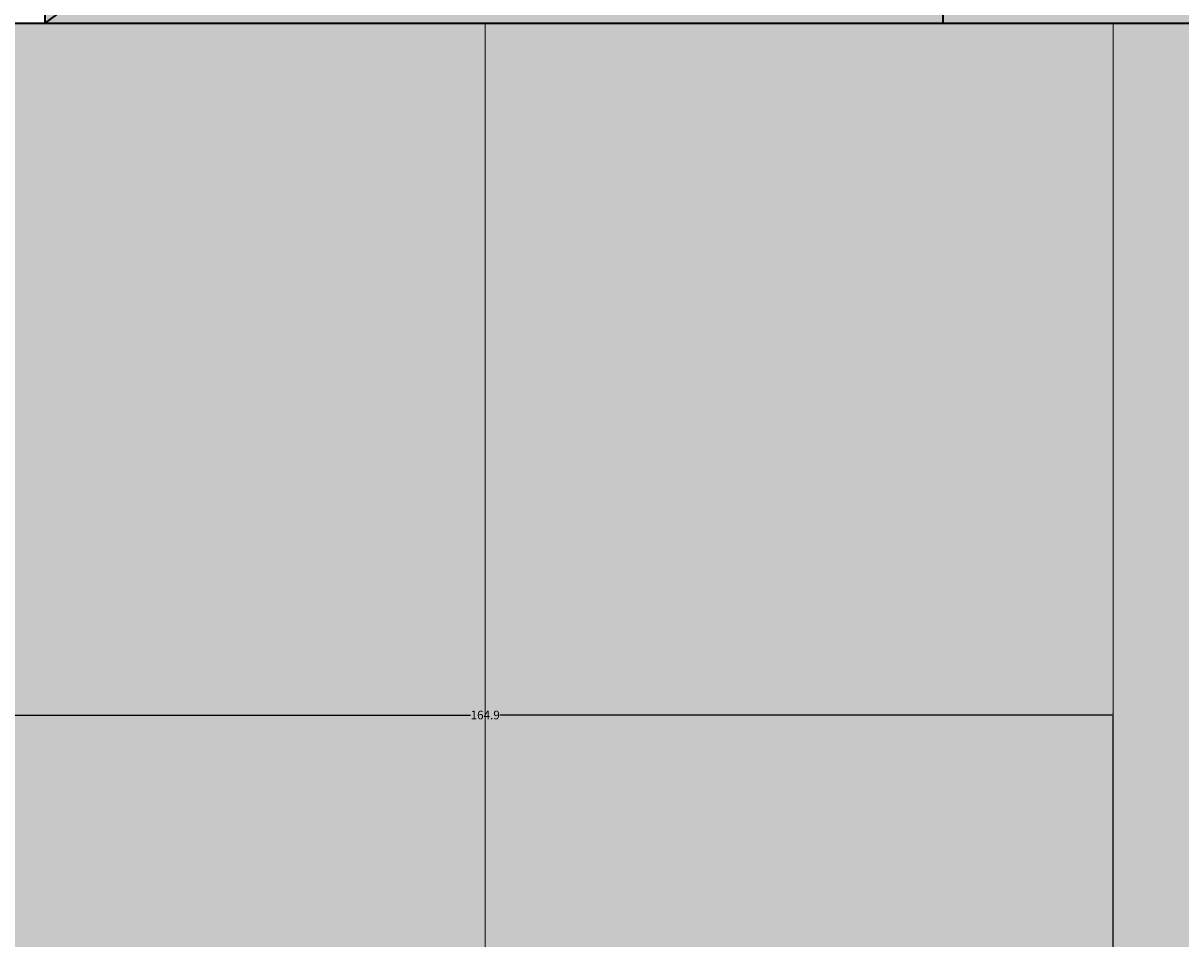
# Model space of a CAD drawing. Units: inches. Extents: x 8 to 634, y 41 to 867.
# Tile 15 of 21: x 141 to 293, y 577 to 698. Entities that reach past the tile are written whole.
import ezdxf

# ---------------------------------------------------------------- set-up
doc = ezdxf.new("R2010")
doc.units = ezdxf.units.IN
doc.header["$MEASUREMENT"] = 0
for name, color, linetype, lineweight in [('A-ANNO-DIMS', 2, 'Continuous', 18), ('A-ELEV-PATT', 252, 'Continuous', 9), ('A-ROOF', 7, 'Continuous', 35), ('A-ROOF-PATT', 8, 'Continuous', 9), ('A-WALL', 7, 'Continuous', 35), ('A-WALL-PANL', 7, 'Continuous', 18), ('A-WALL-PATT', 8, 'Continuous', 9)]:
    doc.layers.add(name, color=color, linetype=linetype, lineweight=lineweight)
doc.styles.get("Standard").update_dxf_attribs({"font": 'arial.ttf'})
doc.dimstyles.get("Standard").update_dxf_attribs({"dimtxt": 1.125, "dimasz": 0.18, "dimexe": 0.18, "dimexo": 0.0625, "dimgap": 0.09, "dimtad": 0, "dimtih": 1, "dimtoh": 1, "dimdec": 4, "dimzin": 0, "dimdsep": 46, "dimlunit": 4, "dimtxsty": 'Standard', "dimcen": 0.09, "dimadec": 0, "dimazin": 0, "dimtfac": 1, "dimtdec": 4, "dimtofl": 0, "dimtmove": 0, "dimatfit": 3, "dimfxl": 1, "dimtolj": 1, "dimtzin": 0, "dimarcsym": 0})

# ---------------------------------------------------------------- blocks, each defined once
blk = doc.blocks.new('*D20')
at = {"layer": 'A-ANNO-DIMS', "color": 0, "lineweight": -2, "transparency": 16777216}
for p, q in [((144.29, 828.98), (9.51, 828.98)), ((9.69, 828.8), (9.69, 454.93)), ((9.69, 79.74), (9.69, 453.6)), ((47.28, 79.56), (9.51, 79.56))]:
    blk.add_line(p, q, dxfattribs=at)
at = {"layer": 'A-ANNO-DIMS', "color": 0, "transparency": 16777216}
for points in [[(9.66, 828.8), (9.72, 828.8), (9.69, 828.98)], [(9.66, 79.74), (9.72, 79.74), (9.69, 79.56)]]:
    blk.add_solid(points, dxfattribs=at)
at = {"layer": 'Defpoints', "color": 0, "transparency": 16777216}
for p in [(9.69, 828.98), (144.36, 828.98), (47.34, 79.56)]:
    blk.add_point(p, dxfattribs=at)
at = {"layer": 'A-ANNO-DIMS', "color": 0, "transparency": 16777216, "insert": (9.69, 454.27), "char_height": 1.125, "attachment_point": 5}
blk.add_mtext('\\A1;749.4', dxfattribs=at)
blk = doc.blocks.new('*D57')
at = {"layer": 'A-ANNO-DIMS', "color": 0, "lineweight": -2, "transparency": 16777216}
for p, q in [((119.71, 569.23), (119.71, 607)), ((119.89, 606.82), (200.22, 606.82)), ((284.43, 606.82), (204.09, 606.82)), ((284.61, 569.23), (284.61, 607))]:
    blk.add_line(p, q, dxfattribs=at)
at = {"layer": 'A-ANNO-DIMS', "color": 0, "transparency": 16777216}
for points in [[(119.89, 606.85), (119.89, 606.79), (119.71, 606.82)], [(284.43, 606.85), (284.43, 606.79), (284.61, 606.82)]]:
    blk.add_solid(points, dxfattribs=at)
at = {"layer": 'Defpoints', "color": 0, "transparency": 16777216}
for p in [(284.61, 606.82), (119.71, 569.17), (284.61, 569.17)]:
    blk.add_point(p, dxfattribs=at)
at = {"layer": 'A-ANNO-DIMS', "color": 0, "transparency": 16777216, "insert": (202.16, 606.82), "char_height": 1.125, "attachment_point": 5}
blk.add_mtext('\\A1;164.9', dxfattribs=at)

msp = doc.modelspace()

# ---------------------------------------------------------------- hatches: boundary and pattern name
at = {"layer": 'A-ELEV-PATT', "transparency": 33554687}
h = msp.add_hatch(color=256, dxfattribs=at)
h.dxf.hatch_style = 1
h.paths.add_polyline_path([(262.2266, 785.231), (144.3564, 697.6655), (262.2266, 697.6655)])
at = {"layer": 'A-ROOF-PATT', "transparency": 33554687}
h = msp.add_hatch(dxfattribs=at)
h.set_pattern_fill('AR-CONC', color=256, scale=2.2, angle=135)
h.paths.add_polyline_path([(262.2266, 828.9821), (144.3564, 828.9821), (144.3564, 697.6655), (262.2266, 785.231), (245.114, 785.231), (245.114, 792.8938), (262.2266, 792.8938)])
h.paths.add_polyline_path([(594.3501, 827.7671), (262.2266, 827.7671), (262.2266, 792.8938), (262.2266, 697.6655), (299.7961, 697.6655), (299.7961, 776.8929), (556.7072, 776.8929), (556.7072, 774.3342), (556.7072, 697.6655), (594.3501, 697.6655)])
at = {"layer": 'A-WALL-PATT', "transparency": 33554687}
h = msp.add_hatch(dxfattribs=at)
h.set_pattern_fill('AR-CONC', color=256, scale=3.2)
h.paths.add_polyline_path([(119.7065, 697.6655), (47.3401, 697.6655), (47.3401, 569.1705), (119.7065, 569.1705)])
h.paths.add_polyline_path([(202.1558, 697.6655), (119.7065, 697.6655), (119.7065, 569.1705), (202.1558, 569.1705)])
h.paths.add_polyline_path([(284.6051, 697.6655), (202.1558, 697.6655), (202.1558, 569.1705), (284.6051, 569.1705)])
h.paths.add_polyline_path([(119.7065, 569.1705), (47.3401, 569.1705), (47.3401, 523.5555), (47.3401, 449.7533), (119.7065, 449.7533)])
h.paths.add_polyline_path([(342.6544, 682.1444), (360.785, 697.6655), (284.6051, 697.6655), (284.6051, 569.1705), (342.6544, 569.1705)])
h.paths.add_polyline_path([(342.6544, 569.1705), (284.6051, 569.1705), (284.6051, 449.7533), (342.6544, 449.7533)])
h.paths.add_polyline_path([(418.2881, 691.978), (418.2881, 697.6655), (360.785, 697.6655), (360.785, 569.1705), (418.2881, 569.1705)])
h.paths.add_polyline_path([(418.2881, 569.1705), (360.785, 569.1705), (360.785, 523.5555), (360.785, 449.7533), (418.2881, 449.7533)])
h.paths.add_polyline_path([(594.3501, 697.6655), (539.0002, 697.6655), (539.0002, 691.978), (539.0002, 569.1705), (594.3501, 569.1705)])
h.paths.add_polyline_path([(594.3501, 523.5555), (594.3501, 569.1705), (539.0002, 569.1705), (539.0002, 451.6305), (594.3501, 451.6305)])
h.paths.add_polyline_path([(594.3501, 451.6305), (539.0002, 451.6305), (539.0002, 391.7598), (594.3501, 391.7598)])
h.paths.add_polyline_path([(594.3501, 391.7598), (539.0002, 391.7598), (539.0002, 276.166), (594.3501, 276.166)])
h.paths.add_polyline_path([(418.2881, 449.7533), (360.785, 449.7533), (360.785, 391.7598), (418.2881, 391.7598)])
h.paths.add_polyline_path([(342.6544, 449.7533), (284.6051, 449.7533), (284.6051, 391.7598), (342.6544, 391.7598)])
h.paths.add_polyline_path([(342.6544, 391.7598), (284.6051, 391.7598), (284.6051, 272.3426), (342.6544, 272.3426)])
h.paths.add_polyline_path([(418.2881, 391.7598), (360.785, 391.7598), (360.785, 272.3426), (418.2881, 272.3426)])
h.paths.add_polyline_path([(418.2881, 272.3426), (360.785, 272.3426), (360.785, 235.5555), (418.2881, 235.5555)])
h.paths.add_polyline_path([(342.6544, 272.3426), (284.6051, 272.3426), (284.6051, 235.5555), (295.0049, 235.5555), (342.6544, 235.5555)])
h.paths.add_polyline_path([(594.3501, 276.166), (539.0002, 276.166), (539.0002, 228.4951), (594.3501, 228.4951)])
h.paths.add_polyline_path([(594.3501, 228.4951), (539.0002, 228.4951), (539.0002, 91.5417), (594.3501, 91.5417)])
h.paths.add_polyline_path([(418.2881, 235.5555), (360.785, 235.5555), (360.785, 91.5417), (418.2881, 91.5417)])
h.paths.add_polyline_path([(284.6051, 272.3426), (119.7065, 272.3426), (119.7065, 235.5555), (284.6051, 235.5555)])
h.paths.add_polyline_path([(119.7065, 272.3426), (47.3401, 272.3426), (47.3401, 235.5555), (47.3401, 91.5555), (63.5448, 91.5555), (63.5448, 227.8036), (268.998, 227.8036), (268.998, 91.5555), (295.0049, 91.5555), (295.0049, 222.583), (271.9787, 222.583), (271.9787, 229.0481), (62.4019, 229.0481), (62.4019, 222.583), (61.1827, 222.583), (61.1827, 235.5555), (119.7065, 235.5555)])
h.paths.add_polyline_path([(119.7065, 391.7598), (47.3401, 391.7598), (47.3401, 379.5555), (47.3401, 272.3426), (119.7065, 272.3426)])
h.paths.add_polyline_path([(119.7065, 449.7533), (47.3401, 449.7533), (47.3401, 391.7598), (119.7065, 391.7598)])
h.paths.add_polyline_path([(202.1558, 449.7533), (119.7065, 449.7533), (119.7065, 391.7598), (202.1558, 391.7598)])
h.paths.add_polyline_path([(284.6051, 449.7533), (202.1558, 449.7533), (202.1558, 391.7598), (284.6051, 391.7598)])

# ---------------------------------------------------------------- linework, layer by layer
at = {"layer": 'A-ROOF'}
for p, q in [((144.3564, 828.9821), (144.3564, 697.6655)), ((262.2266, 828.9821), (262.2266, 697.6655)), ((262.2266, 785.231), (144.3564, 697.6655))]:
    msp.add_line(p, q, dxfattribs=at)
at = {"layer": 'A-WALL'}
msp.add_line((47.3401, 697.6655), (360.785, 697.6655), dxfattribs=at)
at = {"layer": 'A-WALL-PANL'}
for p, q in [((202.1558, 569.1705), (202.1558, 697.6655)), ((284.6051, 569.1705), (284.6051, 697.6655))]:
    msp.add_line(p, q, dxfattribs=at)

# ---------------------------------------------------------------- dimensions: what is measured, and where the dimension line sits
at = {"layer": 'A-ANNO-DIMS'}
dim = msp.add_linear_dim(base=(9.6901, 828.9821), p1=(47.3401, 79.5555), p2=(144.3564, 828.9821), angle=90, dimstyle='Standard', override={"dimdec": 1, "dimlfac": 1, "dimrnd": 0, "dimzin": 0, "dimdsep": 46, "dimlunit": 2}, dxfattribs=at)
dim.commit()
dim.dimension.update_dxf_attribs({"geometry": '*D20', "text_midpoint": (9.6901, 454.2688)})
dim = msp.add_linear_dim(base=(284.6051, 606.8205), p1=(119.7065, 569.1705), p2=(284.6051, 569.1705), dimstyle='Standard', override={"dimdec": 1, "dimlfac": 1, "dimrnd": 0, "dimzin": 0, "dimdsep": 46, "dimlunit": 2}, dxfattribs=at)
dim.commit()
dim.dimension.update_dxf_attribs({"geometry": '*D57', "text_midpoint": (202.1558, 606.8205)})

doc.saveas('drawing.dxf')
